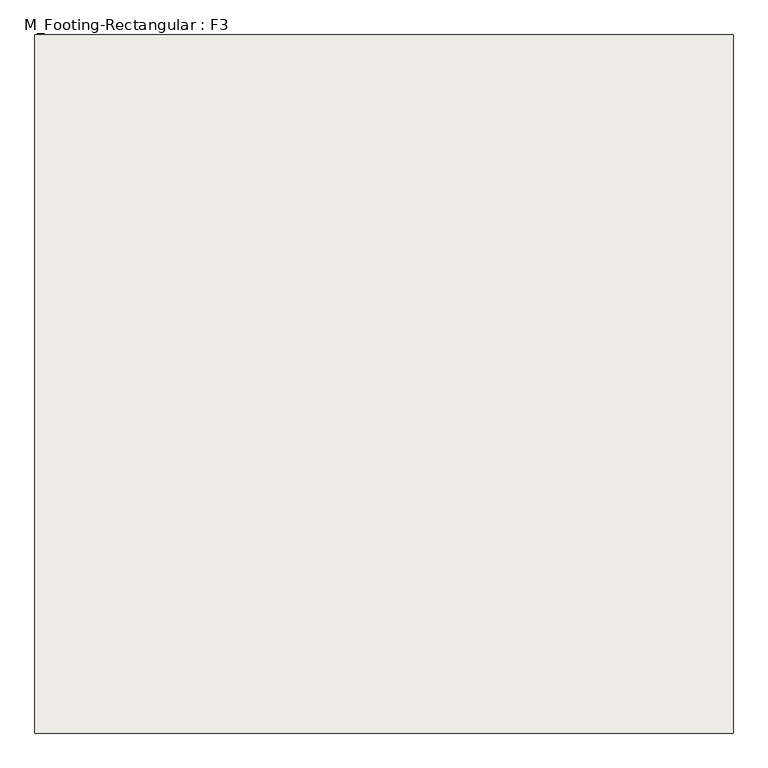
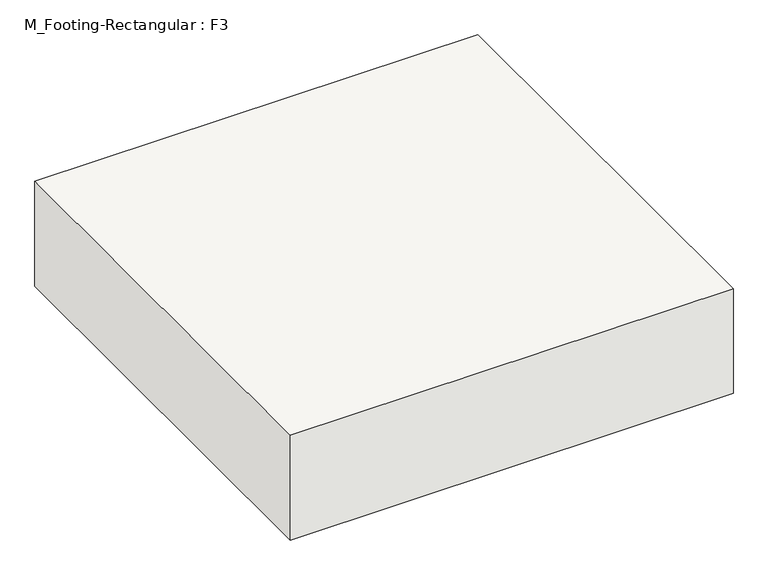
"""IFC4 building model written with IfcOpenShell, lengths in millimetres: slab geometry, M_Footing-Rectangular : F3."""

from ifc_helpers import new_model, si_unit, frame, origin, place, context, project, spatial, polyline, outline, extrude, source, transform, mapped, element, save


def m_footing_rectangular_f3_6d6a3403(model_context):
    return source(origin(), model_context, "Body", "SweptSolid", [
        extrude(outline(polyline([(914.4, 914.4), (914.4, -914.4), (-914.4, -914.4), (-914.4, 914.4), (914.4, 914.4)])), frame((0.0, 0.0, -457.2), z_axis=(0.0, 0.0, 1.0), x_axis=(1.0, 0.0, 0.0)), (0.0, 0.0, 1.0), 457.2),
    ])


if __name__ == "__main__":
    model = new_model("IFC4")
    model_context = context("Model", 3, world=origin())
    ifc_project = project(units=[si_unit("LENGTHUNIT", "METRE", prefix="MILLI")], contexts=[model_context])
    site = spatial("IfcSite", under=ifc_project)
    building = spatial("IfcBuilding", under=site)
    placement = place(None, origin())
    m_footing_rectangular_f3_shape = m_footing_rectangular_f3_6d6a3403(model_context)
    element("IfcSlab", 1, ObjectType="M_Footing-Rectangular : F3", at=placement, inside=building, context=model_context, shape_type="MappedRepresentation", body=[
        mapped(m_footing_rectangular_f3_shape, transform((0.0, 0.0, 0.0), x_axis=(1.0, 0.0, 0.0), y_axis=(0.0, 1.0, 0.0), z_axis=(0.0, 0.0, 1.0))),
    ])
    save(model, "model.ifc")

# Revit data of these elements
# Type "M_Footing-Rectangular : F3"
#   Width = 1828.8 mm
#   Length = 1828.8 mm
#   Foundation Thickness = 457.2 mm
#   Structural Material [instance default] = Concrete, Cast-in-Place gray
#   Assembly Code = ""
# Element 1 (IfcSlab, "M_Footing-Rectangular : F3")
#   Materials on its faces: "Concrete, Cast-in-Place gray"
# Materials
#   "Concrete, Cast-in-Place gray": class "Concrete", colour RGB 192 192 192, transparency 0, Description = "Cast-in-place concrete", Cost = 0
